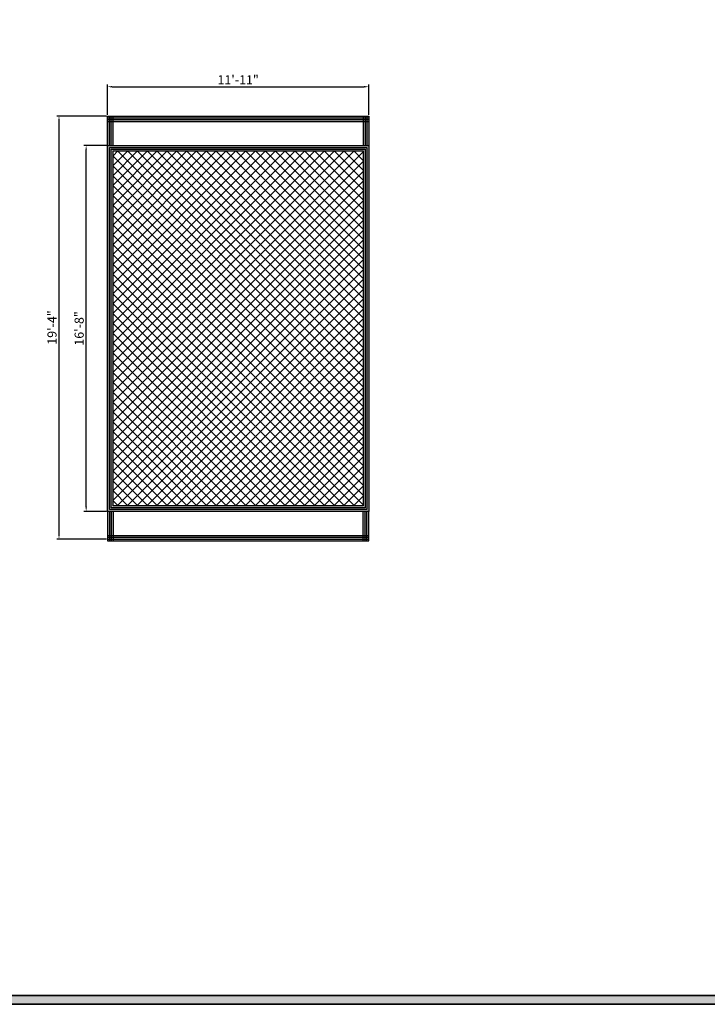
# Model space of a CAD drawing. Units: inches. Extents: x 1804 to 3296, y 909 to 2477.
# Tile 23 of 31: x 2543 to 2920, y 909 to 1449. Entities that reach past the tile are written whole.
import ezdxf

# ---------------------------------------------------------------- set-up
doc = ezdxf.new("R2010")
doc.units = ezdxf.units.IN
for name, color, linetype, lineweight in [('A-ANNO-DIMS', 2, 'Continuous', 18), ('A-ANNO-TTLB', 156, 'Continuous', 35), ('A-WALL-PATT', 10, 'Continuous', 13), ('C-PROP', 7, 'Continuous', 25), ('C-PROP-PATT', 85, 'Continuous', 13)]:
    doc.layers.add(name, color=color, linetype=linetype, lineweight=lineweight)
doc.styles.get("Standard").update_dxf_attribs({"font": 'arial.ttf'})
doc.dimstyles.new('ISO-25', dxfattribs={"dimtxt": 5, "dimasz": 2.5, "dimexe": 1.25, "dimexo": 0.625, "dimtad": 1, "dimdec": 0, "dimlunit": 4, "dimtxsty": 'Standard', "dimcen": 2.5, "dimadec": 0, "dimazin": 0, "dimtfac": 1, "dimtdec": 0, "dimtmove": 0, "dimatfit": 3, "dimfxl": 1, "dimarcsym": 0})

# ---------------------------------------------------------------- blocks, each defined once
blk = doc.blocks.new('*D40')
at = {"layer": 'A-ANNO-DIMS', "color": 0, "lineweight": -2, "transparency": 16777216}
for p, q in [((2590.91, 1395.84), (2563.72, 1395.84)), ((2564.97, 1166.73), (2564.97, 1393.34)), ((2590.91, 1164.23), (2563.72, 1164.23))]:
    blk.add_line(p, q, dxfattribs=at)
at = {"layer": 'A-ANNO-DIMS', "color": 0, "lineweight": 100, "transparency": 16777216}
for points in [[(2564.55, 1393.34), (2565.38, 1393.34), (2564.97, 1395.84)], [(2564.55, 1166.73), (2565.38, 1166.73), (2564.97, 1164.23)]]:
    blk.add_solid(points, dxfattribs=at)
at = {"layer": 'Defpoints', "color": 0, "lineweight": 100, "transparency": 16777216}
for p in [(2564.97, 1395.84), (2591.54, 1395.84), (2591.54, 1164.23)]:
    blk.add_point(p, dxfattribs=at)
at = {"layer": 'A-ANNO-DIMS', "color": 0, "transparency": 16777216, "insert": (2561.79, 1280.03), "char_height": 5, "attachment_point": 5, "rotation": 90}
blk.add_mtext('19\'-4"', dxfattribs=at)
blk = doc.blocks.new('*D41')
at = {"layer": 'A-ANNO-DIMS', "color": 0, "lineweight": -2, "transparency": 16777216}
for p, q in [((2590.91, 1379.68), (2578.58, 1379.68)), ((2579.83, 1181.88), (2579.83, 1377.18)), ((2590.91, 1179.38), (2578.58, 1179.38))]:
    blk.add_line(p, q, dxfattribs=at)
at = {"layer": 'A-ANNO-DIMS', "color": 0, "lineweight": 100, "transparency": 16777216}
for points in [[(2579.41, 1377.18), (2580.24, 1377.18), (2579.83, 1379.68)], [(2579.41, 1181.88), (2580.24, 1181.88), (2579.83, 1179.38)]]:
    blk.add_solid(points, dxfattribs=at)
at = {"layer": 'Defpoints', "color": 0, "lineweight": 100, "transparency": 16777216}
for p in [(2579.83, 1379.68), (2591.54, 1379.68), (2591.54, 1179.38)]:
    blk.add_point(p, dxfattribs=at)
at = {"layer": 'A-ANNO-DIMS', "color": 0, "transparency": 16777216, "insert": (2576.65, 1279.53), "char_height": 5, "attachment_point": 5, "rotation": 90}
blk.add_mtext('16\'-8"', dxfattribs=at)
blk = doc.blocks.new('*D42')
at = {"layer": 'A-ANNO-DIMS', "color": 0, "lineweight": -2, "transparency": 16777216}
for p, q in [((2591.54, 1396.47), (2591.54, 1413.1)), ((2734.5, 1396.47), (2734.5, 1413.1)), ((2594.04, 1411.85), (2732, 1411.85))]:
    blk.add_line(p, q, dxfattribs=at)
at = {"layer": 'A-ANNO-DIMS', "color": 0, "lineweight": 100, "transparency": 16777216}
for points in [[(2594.04, 1412.27), (2594.04, 1411.44), (2591.54, 1411.85)], [(2732, 1412.27), (2732, 1411.44), (2734.5, 1411.85)]]:
    blk.add_solid(points, dxfattribs=at)
at = {"layer": 'Defpoints', "color": 0, "lineweight": 100, "transparency": 16777216}
for p in [(2734.5, 1411.85), (2591.54, 1395.84), (2734.5, 1395.84)]:
    blk.add_point(p, dxfattribs=at)
at = {"layer": 'A-ANNO-DIMS', "color": 0, "transparency": 16777216, "insert": (2663.02, 1414.99), "char_height": 5, "attachment_point": 5}
blk.add_mtext('11\'-11"', dxfattribs=at)

msp = doc.modelspace()

# ---------------------------------------------------------------- hatches: boundary and pattern name
at = {"layer": 'A-ANNO-TTLB'}
h = msp.add_hatch(color=256, dxfattribs=at)
h.dxf.hatch_style = 1
h.paths.add_polyline_path([(3294.53, 2476.54), (1803.79, 2476.54), (1805.43, 909.47), (3296.17, 909.47)])
h.paths.add_polyline_path([(1811, 914.33), (1812.79, 2467.54), (3285.53, 2467.54), (3283.74, 914.33)], flags=16)
h.paths.add_polyline_path([(1925.58, 1062.77), (1925.58, 1138.07), (1925.58, 1539.88), (1925.58, 1793.38), (1925.58, 1830.04), (2325.54, 1830.04), (2325.54, 1793.38), (2325.54, 1586.42), (2325.54, 1138.07), (2325.54, 1062.77)], flags=0)
h.paths.add_polyline_path([(1997.22, 1029.4), (2008.85, 1037.96), (2008.85, 1020.84)], flags=0)
h.paths.add_polyline_path([(1934.58, 1138.07), (1934.58, 1147.07), (2078.77, 1147.07), (2078.77, 1138.07), (2060.94, 1138.07)], flags=0)
h.paths.add_polyline_path([(1944.35, 1138.07), (1944.35, 1147.07), (2056.05, 1147.07), (2056.05, 1138.07)], flags=0)
h.paths.add_polyline_path([(2222.24, 1037.96), (2233.87, 1029.4), (2222.24, 1020.84)], flags=0)
h.paths.add_polyline_path([(2061.94, 1139.07), (2061.94, 1146.07), (2077.77, 1146.07), (2077.77, 1139.07)], flags=0)
h.paths.add_polyline_path([(2149.58, 1138.07), (2149.58, 1269.44), (2158.58, 1269.44), (2158.58, 1326.69), (2149.58, 1326.69), (2149.58, 1340.94), (2139.6, 1340.94), (2139.6, 1434.25), (2149.58, 1434.25), (2149.58, 1447.36), (2158.58, 1447.36), (2158.58, 1423.87), (2158.58, 1408.06), (2198.46, 1408.06), (2198.46, 1412.56), (2282.65, 1412.56), (2282.65, 1465.94), (2316.54, 1465.94), (2316.54, 1590.92), (2192.86, 1590.92), (2192.86, 1595.3), (2291.17, 1595.3), (2291.17, 1590.92), (2316.54, 1590.92), (2316.54, 1784.38), (2300.24, 1784.38), (2300.24, 1757.47), (2268, 1757.47), (2268, 1681.04), (2180.87, 1681.04), (2180.87, 1757.47), (2148.63, 1757.47), (2148.63, 1784.38), (2119.08, 1784.38), (2119.08, 1585.58), (2114.58, 1585.58), (2114.58, 1784.38), (2064.11, 1784.38), (2046.28, 1784.38), (2046.28, 1760.38), (1958.58, 1760.38), (1958.58, 1664.38), (1934.58, 1664.38), (1934.58, 1784.38), (1934.58, 1793.38), (2046.28, 1793.38), (2064.11, 1793.38), (2119.08, 1793.38), (2230.78, 1793.38), (2230.78, 1784.38), (2268, 1784.38), (2300.24, 1784.38), (2316.54, 1784.38), (2316.54, 1590.92), (2316.54, 1373.73), (2316.54, 1138.07)], flags=0)
h.paths.add_polyline_path([(2209.19, 1166.63), (2209.19, 1175.63), (2158.58, 1175.63), (2209.19, 1223.63), (2209.19, 1231.63), (2183.88, 1231.63), (2183.88, 1301.66), (2242.59, 1301.66), (2242.59, 1326.69), (2316.54, 1326.69), (2272.59, 1271.63), (2272.59, 1223.63), (2316.54, 1175.63), (2272.59, 1175.63), (2272.59, 1166.63)], flags=0)
h.paths.add_polyline_path([(1947.77, 1345.22), (1947.77, 1457.48), (1991.2, 1457.48), (1991.2, 1451.7), (1991.2, 1352.18), (1991.2, 1345.22)], flags=0)
h.paths.add_polyline_path([(2209.19, 1271.63), (2262.59, 1271.63), (2262.59, 1311.85), (2272.59, 1301.66), (2272.59, 1271.63), (2269.92, 1269.63), (2270.59, 1269.63), (2270.59, 1225.63), (2211.19, 1225.63), (2211.19, 1269.63), (2211.86, 1269.63)], flags=0)
h.paths.add_polyline_path([(2000.34, 1378.21), (2000.34, 1429.71), (2025.22, 1429.71), (2025.22, 1378.21)], flags=0)
h.paths.add_polyline_path([(2001.34, 1379.21), (2001.34, 1428.71), (2024.22, 1428.71), (2024.22, 1379.21)], flags=0)
h.paths.add_polyline_path([(2012.34, 1390.21), (2012.34, 1417.71), (2013.22, 1417.71), (2013.22, 1390.21)], flags=0)
h.paths.add_polyline_path([(2237.56, 1331.19), (2237.56, 1340.18), (2238.62, 1340.18), (2238.62, 1386.84), (2241.04, 1386.84), (2242.06, 1386.84), (2242.06, 1408.06), (2316.54, 1331.19)], flags=0)
h.paths.add_polyline_path([(1953.73, 1464.35), (1953.73, 1498.59), (1981.74, 1498.59), (1981.74, 1464.35)], flags=0)
h.paths.add_polyline_path([(1987.63, 1462.08), (1987.63, 1500.95), (2104.07, 1500.95), (2104.07, 1462.08), (2099.27, 1462.08), (1993.6, 1462.08)], flags=0)
h.paths.add_polyline_path([(1956.06, 1481.47, -1), (1979.41, 1481.47, -1)], flags=0)
edge = h.paths.add_edge_path(flags=0)
edge.add_ellipse((2299.53, 1438.37), major_axis=(0.31, 21.36), ratio=0.670333, start_angle=0, end_angle=360)
h.paths.add_polyline_path([(2297.39, 1438.37, -1), (2301.67, 1438.37, -1)], flags=0)
h.paths.add_polyline_path([(2591.54, 1163.23), (2591.54, 1179.38), (2591.54, 1379.68), (2591.54, 1395.84), (2734.5, 1395.84), (2734.5, 1379.68), (2734.5, 1179.38), (2734.5, 1163.23)], flags=0)
h.paths.add_polyline_path([(2592.54, 1164.23), (2592.54, 1166.23), (2733.5, 1166.23), (2733.5, 1164.23)], flags=0)
h.paths.add_polyline_path([(2592.54, 1180.38), (2592.54, 1378.68), (2733.5, 1378.68), (2733.5, 1180.38)], flags=0)
h.paths.add_polyline_path([(2593.54, 1181.38), (2593.54, 1377.68), (2732.5, 1377.68), (2732.5, 1181.38)], flags=0)
h.paths.add_polyline_path([(2594.54, 1182.38), (2594.54, 1376.68), (2731.5, 1376.68), (2731.5, 1182.38)], flags=0)
h.paths.add_polyline_path([(1936.95, 1697.46), (1936.95, 1736.46), (1955.41, 1736.46), (1955.41, 1697.46)], flags=0)
h.paths.add_polyline_path([(1938.48, 1718.36), (1938.48, 1734.92), (1953.65, 1734.92), (1953.65, 1718.36)], flags=0)
h.paths.add_polyline_path([(1944.75, 1726.64, -1), (1947.37, 1726.64, -1)], flags=0)
h.paths.add_polyline_path([(2592.54, 1394.84), (2733.5, 1394.84), (2733.5, 1392.84), (2592.54, 1392.84)], flags=0)
h.paths.add_polyline_path([(1976.61, 1762.5), (1976.61, 1781.44), (2012.79, 1781.44), (2012.79, 1762.5)], flags=0)
h.paths.add_polyline_path([(1979.57, 1771.97, -1), (1991.39, 1771.97, -1)], flags=0)
h.paths.add_polyline_path([(1995.36, 1771.97, -1), (2007.18, 1771.97, -1)], flags=0)
h.paths.add_polyline_path([(2251.51, 1744.53), (2268, 1730.05), (2251.51, 1730.05)], flags=0)
h.paths.add_polyline_path([(2047.28, 1785.38), (2047.28, 1792.38), (2063.11, 1792.38), (2063.11, 1785.38)], flags=0)
h.paths.add_polyline_path([(2155.08, 1770.92, -1), (2174.42, 1770.92, -1)], flags=0)
h.paths.add_polyline_path([(2188.59, 1758.27), (2188.59, 1772.81), (2222.3, 1772.81), (2222.3, 1758.27)], flags=0)
h.paths.add_polyline_path([(2223.97, 1758.27), (2223.97, 1772.81), (2257.68, 1772.81), (2257.68, 1758.27)], flags=0)
h.paths.add_polyline_path([(2274.45, 1770.92, -1), (2293.8, 1770.92, -1)], flags=0)
h.paths.add_polyline_path([(2591.54, 1582.09), (2591.54, 1782.39), (2734.5, 1782.39), (2734.5, 1582.09)], flags=0)
h.paths.add_polyline_path([(2592.54, 1583.09), (2592.54, 1781.39), (2733.5, 1781.39), (2733.5, 1583.09)], flags=0)
h.paths.add_polyline_path([(2593.54, 1584.09), (2593.54, 1780.39), (2732.5, 1780.39), (2732.5, 1584.09)], flags=0)
h.paths.add_polyline_path([(2594.54, 1585.09), (2594.54, 1779.39), (2731.5, 1779.39), (2731.5, 1585.09)], flags=0)
h.paths.add_polyline_path([(1922.17, 1978.79), (1922.17, 2295.08), (1922.17, 2296.08), (2115.67, 2296.08), (2115.67, 2384.31), (2115.67, 2385.31), (2322.12, 2385.31), (2323.12, 2385.31), (2323.12, 1979.79), (2323.12, 1978.79), (1923.17, 1978.79)], flags=0)
h.paths.add_polyline_path([(1922.17, 1978.79), (1922.17, 2051.31), (1922.17, 2214.86), (1922.17, 2296.08), (2115.67, 2296.08), (2115.67, 2385.31), (2323.12, 2385.31), (2323.12, 2280.42), (2323.12, 1978.79), (2115.67, 1978.79)], flags=0)
h.paths.add_polyline_path([(1923.17, 1979.79), (1923.17, 2050.31), (2115.67, 2050.31), (2115.67, 2051.31), (1923.17, 2051.31), (1923.17, 2213.86), (1923.17, 2214.86), (1923.17, 2295.08), (1990.02, 2295.08), (1990.02, 2214.86), (1991.02, 2214.86), (1991.02, 2295.08), (2115.67, 2295.08), (2115.67, 1979.79), (2116.67, 1979.79), (2116.67, 2304.18), (2116.67, 2384.31), (2322.12, 2384.31), (2322.12, 2280.42), (2322.12, 1979.79), (2115.67, 1979.79)], flags=0)
h.paths.add_polyline_path([(2972.46, 1192.5), (2972.46, 1196.92), (2995.47, 1196.92), (2995.47, 1255.47), (2995.09, 1255.47), (2987.42, 1249.39), (2980.08, 1255.47), (2978.05, 1255.47), (2978.05, 1257.24), (2995.47, 1257.24), (2995.47, 1261.58), (3015.37, 1261.58), (3015.37, 1333.28), (3015.37, 1414.4), (3032.82, 1414.4), (3032.82, 1333.28), (3032.82, 1261.58), (3052.66, 1261.58), (3052.66, 1255.47), (3079.86, 1255.47), (3078.72, 1254.57), (3081.47, 1252.29), (3078.56, 1249.99), (3075.81, 1252.26), (3072.57, 1249.69), (3070.36, 1251.52), (3067.67, 1249.39), (3060.34, 1255.47), (3052.66, 1255.47), (3052.66, 1196.92), (3054.58, 1196.92), (3074, 1196.92), (3074, 1192.5), (3052.66, 1192.5), (2995.47, 1192.5)], flags=0)
h.paths.add_polyline_path([(2490.75, 1979.27), (2490.75, 1980.27), (2596.87, 1980.27), (2596.87, 2051.8), (2596.87, 2052.8), (2596.87, 2216.35), (2596.87, 2297.57), (2717.32, 2297.57), (2710.57, 2305.62), (2724.07, 2305.62), (2717.32, 2297.57), (2782.37, 2297.57), (2782.37, 2395.8), (3006.82, 2395.8), (3006.82, 1981.27), (3093.73, 1981.27), (3093.73, 1980.27), (3047.51, 1980.27), (3046.37, 1979.37), (3049.11, 1977.1), (3046.2, 1974.79), (3043.46, 1977.07), (3040.21, 1974.49), (3038, 1976.32), (3035.32, 1974.2), (3027.98, 1980.27), (2871.83, 1980.27), (2871.83, 1981.27), (2791.37, 1981.27), (2791.37, 2050.8), (2597.87, 2050.8), (2597.87, 1980.27), (2597.87, 1979.27), (2546.27, 1979.27), (2545.12, 1978.37), (2547.87, 1976.1), (2544.96, 1973.79), (2542.22, 1976.07), (2538.97, 1973.49), (2536.76, 1975.32), (2534.07, 1973.2), (2526.74, 1979.27)], flags=0)
h.paths.add_polyline_path([(2597.87, 2051.8), (2606.87, 2051.8), (2606.87, 2258.39), (2597.87, 2258.39), (2597.87, 2296.57), (2606.87, 2296.57), (2606.87, 2262.39), (2782.37, 2262.39), (2782.37, 2296.57), (2790.37, 2296.57), (2790.37, 2262.39), (2791.37, 2262.39), (2791.37, 2305.67), (2791.37, 2385.8), (2996.82, 2385.8), (2996.82, 2339.85), (3006.82, 2339.85), (3006.82, 2250.12), (2997.82, 2250.12), (2997.82, 1981.27), (2996.82, 1981.27), (2872.83, 1981.27), (2872.83, 1991.8), (2871.83, 1991.8), (2871.83, 2050.8), (2790.37, 2050.8), (2597.87, 2050.8)], flags=0)
h.paths.add_polyline_path([(2179.93, 2153.92), (2179.93, 2353.97), (2259.98, 2353.97), (2259.98, 2153.92)], flags=0)
h.paths.add_polyline_path([(2180.93, 2154.92), (2180.93, 2352.97), (2258.98, 2352.97), (2258.98, 2154.92)], flags=0)
h.paths.add_polyline_path([(2960.87, 1608.49), (2960.87, 1753.62), (3070.9, 1753.62), (3070.9, 1608.49)], flags=0)
h.paths.add_polyline_path([(2961.87, 1609.49), (2961.87, 1752.62), (3069.9, 1752.62), (3069.9, 1609.49)], flags=0)
h.paths.add_polyline_path([(2962.87, 1610.49), (2962.87, 1751.62), (3068.9, 1751.62), (3068.9, 1610.49)], flags=0)
h.paths.add_polyline_path([(2963.87, 1611.49), (2963.87, 1750.62), (3067.9, 1750.62), (3067.9, 1611.49)], flags=0)
h.paths.add_polyline_path([(2782.37, 2051.8), (2782.37, 2216.32), (2791.37, 2216.32), (2791.37, 2051.8), (2872.83, 2051.8), (2872.83, 2068.56), (2884.67, 2068.56), (2884.67, 2085.33), (2896.51, 2085.33), (2896.51, 2102.09), (2908.36, 2102.09), (2908.36, 2118.85), (2920.2, 2118.85), (2920.2, 2135.62), (2932.05, 2135.62), (2932.05, 2145.3), (2925.08, 2145.3), (2925.08, 2203.2), (2996.82, 2203.2), (2996.82, 2145.3), (2953.82, 2145.3), (2872.83, 2051.8), (2790.37, 2051.8)], flags=0)
h.paths.add_polyline_path([(2717.32, 2238.65), (2710.57, 2246.7), (2724.07, 2246.7)], flags=0)
h.paths.add_polyline_path([(2003.09, 1122.79), (2017.16, 1122.79), (2017.16, 1138.74), (2003.09, 1138.74)], flags=8)
h.paths.add_polyline_path([(2174.76, 1792.72), (2188.83, 1792.72), (2188.83, 1808.66), (2174.76, 1808.66)], flags=8)
h.paths.add_polyline_path([(1987.95, 1792.51), (2002.02, 1792.51), (2002.02, 1808.45), (1987.95, 1808.45)], flags=8)
h.paths.add_polyline_path([(2148.79, 1289.26), (2160.46, 1289.26), (2160.46, 1305.2), (2148.79, 1305.2)], flags=8)
h.paths.add_polyline_path([(2115.36, 1133.57), (2127.04, 1133.57), (2127.04, 1149.51), (2115.36, 1149.51)], flags=8)
h.paths.add_polyline_path([(2237.58, 1421.48), (2249.25, 1421.48), (2249.25, 1437.43), (2237.58, 1437.43)], flags=8)
h.paths.add_polyline_path([(2134.99, 1584.32), (2146.66, 1584.32), (2146.66, 1600.26), (2134.99, 1600.26)], flags=8)
h.paths.add_polyline_path([(2101.95, 1557.31), (2113.62, 1557.31), (2113.62, 1573.25), (2101.95, 1573.25)], flags=8)
h.paths.add_polyline_path([(2937.85, 1156.77), (3120.41, 1156.77), (3120.41, 1185.72), (2937.85, 1185.72)], flags=8)
h.paths.add_polyline_path([(2980.71, 1786.71), (3050.06, 1786.71), (3050.06, 1802.66), (2980.71, 1802.66)], flags=8)
h.paths.add_polyline_path([(2869.28, 1661.96), (2938.62, 1661.96), (2938.62, 1690.8), (2869.28, 1690.8)], flags=8)
h.paths.add_polyline_path([(3092.27, 1674.86), (3161.62, 1674.86), (3161.62, 1690.8), (3092.27, 1690.8)], flags=8)
h.paths.add_polyline_path([(2980.71, 1674.86), (3050.06, 1674.86), (3050.06, 1690.8), (2980.71, 1690.8)], flags=8)
h.paths.add_polyline_path([(2649.07, 1678.23), (2674.53, 1678.23), (2674.53, 1714.76), (2649.07, 1714.76)], flags=8)
h.paths.add_polyline_path([(2530.84, 1981.63), (2549.13, 1981.63), (2549.13, 1997.57), (2530.84, 1997.57)], flags=8)
h.paths.add_polyline_path([(3031.29, 1981.77), (3049.58, 1981.77), (3049.58, 1997.71), (3031.29, 1997.71)], flags=8)
h.paths.add_polyline_path([(2715.38, 1911.9), (2851.54, 1911.9), (2851.54, 1940.85), (2715.38, 1940.85)], flags=8)
h.paths.add_polyline_path([(2015.23, 1927.36), (2205.42, 1927.36), (2205.42, 1956.3), (2015.23, 1956.3)], flags=8)
h.paths.add_polyline_path([(2671.84, 2057.84), (2702.75, 2057.84), (2702.75, 2073.79), (2671.84, 2073.79)], flags=8)
h.paths.add_polyline_path([(2678.5, 2316.52), (2765.26, 2316.52), (2765.26, 2332.46), (2678.5, 2332.46)], flags=8)
h.paths.add_polyline_path([(2678.48, 2271.96), (2736.41, 2271.96), (2736.41, 2287.9), (2678.48, 2287.9)], flags=8)
h.paths.add_polyline_path([(2019.2, 972.79), (2243.21, 972.79), (2243.21, 1001.74), (2019.2, 1001.74)], flags=8)
h.paths.add_polyline_path([(2097.06, 1021.56), (2132.16, 1021.56), (2132.16, 1037.51), (2097.06, 1037.51)], flags=8)
h.paths.add_polyline_path([(2182.47, 1360.48), (2207.35, 1360.48), (2207.35, 1376.42), (2182.47, 1376.42)], flags=8)
h.paths.add_polyline_path([(2261.12, 1361.77), (2295.01, 1361.77), (2295.01, 1377.71), (2261.12, 1377.71)], flags=8)
h.paths.add_polyline_path([(2245.75, 1511.51), (2278.44, 1511.51), (2278.44, 1527.46), (2245.75, 1527.46)], flags=8)
h.paths.add_polyline_path([(1991.16, 1296.29), (2060.51, 1296.29), (2060.51, 1312.23), (1991.16, 1312.23)], flags=8)
h.paths.add_polyline_path([(2187, 1651.35), (2246.71, 1651.35), (2246.71, 1667.29), (2187, 1667.29)], flags=8)
h.paths.add_polyline_path([(1976.49, 1684.81), (2068.63, 1684.81), (2068.63, 1700.76), (1976.49, 1700.76)], flags=8)
at = {"layer": 'A-WALL-PATT'}
h = msp.add_hatch(color=256, dxfattribs=at)
h.dxf.hatch_style = 1
h.paths.add_polyline_path([(2158.58, 1275.49), (2155.29, 1275.49), (2149.58, 1275.49), (2149.58, 1269.44), (2158.58, 1269.44)])
h.paths.add_polyline_path([(2158.58, 1326.69), (2149.58, 1326.69), (2149.58, 1319.33), (2155.29, 1319.33), (2158.58, 1319.33)])
h.paths.add_polyline_path([(2158.58, 1402.2), (2158.58, 1423.87), (2158.58, 1447.36), (2149.58, 1447.36), (2149.58, 1423.87), (2149.58, 1340.94), (2149.58, 1326.69), (2158.58, 1326.69), (2158.58, 1354.23)])
h.paths.add_polyline_path([(1965.87, 1658.79), (1965.87, 1679.09), (1955.57, 1679.09), (1955.57, 1658.79)], flags=9)
h.paths.add_polyline_path([(2293.18, 1677.29), (2293.18, 1697.58), (2282.88, 1697.58), (2282.88, 1677.29)], flags=9)
h.paths.add_polyline_path([(2271.13, 1545.23), (2287.53, 1545.23), (2287.53, 1555.53), (2271.13, 1555.53)], flags=9)
h.paths.add_polyline_path([(2303.26, 1488.52), (2303.26, 1508.82), (2292.95, 1508.82), (2292.95, 1488.52)], flags=9)
h.paths.add_polyline_path([(2271.13, 1393.15), (2287.53, 1393.15), (2287.53, 1403.45), (2271.13, 1403.45)], flags=9)
h.paths.add_polyline_path([(2306.48, 1361.45), (2306.48, 1377.86), (2296.18, 1377.86), (2296.18, 1361.45)], flags=9)
h.paths.add_polyline_path([(2189.9, 1340.62), (2206.31, 1340.62), (2206.31, 1350.92), (2189.9, 1350.92)], flags=9)
h.paths.add_polyline_path([(2174.54, 1361.45), (2174.54, 1377.86), (2164.23, 1377.86), (2164.23, 1361.45)], flags=9)
h.paths.add_polyline_path([(2304.24, 1240.8), (2304.24, 1261.09), (2293.94, 1261.09), (2293.94, 1240.8)], flags=9)
h.paths.add_polyline_path([(2227.19, 1188.73), (2247.49, 1188.73), (2247.49, 1199.03), (2227.19, 1199.03)], flags=9)
h.paths.add_polyline_path([(2181.93, 1144.21), (2181.93, 1160.62), (2171.63, 1160.62), (2171.63, 1144.21)], flags=9)
h.paths.add_polyline_path([(1968.21, 1333.34), (1968.21, 1353.64), (1957.91, 1353.64), (1957.91, 1333.34)], flags=9)
h.paths.add_polyline_path([(2029.78, 1203.53), (2053.95, 1203.53), (2053.95, 1213.83), (2029.78, 1213.83)], flags=9)
h.paths.add_polyline_path([(2576.51, 1671.88), (2576.51, 1692.17), (2566.21, 1692.17), (2566.21, 1671.88)], flags=9)
h.paths.add_polyline_path([(2566.99, 1269.67), (2566.99, 1289.96), (2556.68, 1289.96), (2556.68, 1269.67)], flags=9)
h.paths.add_polyline_path([(2581.85, 1269.17), (2581.85, 1289.46), (2571.54, 1289.46), (2571.54, 1269.17)], flags=9)
h.paths.add_polyline_path([(2650.71, 1409.75), (2674.89, 1409.75), (2674.89, 1420.05), (2650.71, 1420.05)], flags=9)
h.paths.add_polyline_path([(2003.09, 1122.79), (2017.16, 1122.79), (2017.16, 1138.74), (2003.09, 1138.74)], flags=9)
h.paths.add_polyline_path([(2174.76, 1792.72), (2188.83, 1792.72), (2188.83, 1808.66), (2174.76, 1808.66)], flags=9)
h.paths.add_polyline_path([(1987.95, 1792.51), (2002.02, 1792.51), (2002.02, 1808.45), (1987.95, 1808.45)], flags=9)
h.paths.add_polyline_path([(2148.79, 1289.26), (2160.46, 1289.26), (2160.46, 1305.2), (2148.79, 1305.2)], flags=9)
h.paths.add_polyline_path([(2115.36, 1133.57), (2127.04, 1133.57), (2127.04, 1149.51), (2115.36, 1149.51)], flags=9)
h.paths.add_polyline_path([(2237.58, 1421.48), (2249.25, 1421.48), (2249.25, 1437.43), (2237.58, 1437.43)], flags=9)
h.paths.add_polyline_path([(2134.99, 1584.32), (2146.66, 1584.32), (2146.66, 1600.26), (2134.99, 1600.26)], flags=9)
h.paths.add_polyline_path([(2101.95, 1557.31), (2113.62, 1557.31), (2113.62, 1573.25), (2101.95, 1573.25)], flags=9)
h.paths.add_polyline_path([(2937.85, 1156.77), (3120.41, 1156.77), (3120.41, 1185.72), (2937.85, 1185.72)], flags=9)
h.paths.add_polyline_path([(2980.71, 1786.71), (3050.06, 1786.71), (3050.06, 1802.66), (2980.71, 1802.66)], flags=9)
h.paths.add_polyline_path([(2869.28, 1661.96), (2938.62, 1661.96), (2938.62, 1690.8), (2869.28, 1690.8)], flags=9)
h.paths.add_polyline_path([(3092.27, 1674.86), (3161.62, 1674.86), (3161.62, 1690.8), (3092.27, 1690.8)], flags=9)
h.paths.add_polyline_path([(2980.71, 1674.86), (3050.06, 1674.86), (3050.06, 1690.8), (2980.71, 1690.8)], flags=9)
h.paths.add_polyline_path([(2649.07, 1678.23), (2674.53, 1678.23), (2674.53, 1714.76), (2649.07, 1714.76)], flags=9)
h.paths.add_polyline_path([(2530.84, 1981.63), (2549.13, 1981.63), (2549.13, 1997.57), (2530.84, 1997.57)], flags=9)
h.paths.add_polyline_path([(3031.29, 1981.77), (3049.58, 1981.77), (3049.58, 1997.71), (3031.29, 1997.71)], flags=9)
h.paths.add_polyline_path([(2715.38, 1911.9), (2851.54, 1911.9), (2851.54, 1940.85), (2715.38, 1940.85)], flags=9)
h.paths.add_polyline_path([(2015.23, 1927.36), (2205.42, 1927.36), (2205.42, 1956.3), (2015.23, 1956.3)], flags=9)
h.paths.add_polyline_path([(2671.84, 2057.84), (2702.75, 2057.84), (2702.75, 2073.79), (2671.84, 2073.79)], flags=9)
h.paths.add_polyline_path([(2678.5, 2316.52), (2765.26, 2316.52), (2765.26, 2332.46), (2678.5, 2332.46)], flags=9)
h.paths.add_polyline_path([(2678.48, 2271.96), (2736.41, 2271.96), (2736.41, 2287.9), (2678.48, 2287.9)], flags=9)
h.paths.add_polyline_path([(2019.2, 972.79), (2243.21, 972.79), (2243.21, 1001.74), (2019.2, 1001.74)], flags=9)
h.paths.add_polyline_path([(2097.06, 1021.56), (2132.16, 1021.56), (2132.16, 1037.51), (2097.06, 1037.51)], flags=9)
h.paths.add_polyline_path([(2182.47, 1360.48), (2207.35, 1360.48), (2207.35, 1376.42), (2182.47, 1376.42)], flags=9)
h.paths.add_polyline_path([(2261.12, 1361.77), (2295.01, 1361.77), (2295.01, 1377.71), (2261.12, 1377.71)], flags=9)
h.paths.add_polyline_path([(2245.75, 1511.51), (2278.44, 1511.51), (2278.44, 1527.46), (2245.75, 1527.46)], flags=9)
h.paths.add_polyline_path([(1991.16, 1296.29), (2060.51, 1296.29), (2060.51, 1312.23), (1991.16, 1312.23)], flags=9)
h.paths.add_polyline_path([(2187, 1651.35), (2246.71, 1651.35), (2246.71, 1667.29), (2187, 1667.29)], flags=9)
h.paths.add_polyline_path([(1976.49, 1684.81), (2068.63, 1684.81), (2068.63, 1700.76), (1976.49, 1700.76)], flags=9)
at = {"layer": 'C-PROP-PATT'}
h = msp.add_hatch(color=256, dxfattribs=at)
h.dxf.hatch_style = 1
h.paths.add_polyline_path([(2734.5, 1392.84), (2733.5, 1392.84), (2733.5, 1379.68), (2734.5, 1379.68)])
h.paths.add_polyline_path([(2733.5, 1392.84), (2732.5, 1392.84), (2732.5, 1379.68), (2733.5, 1379.68)])
h.paths.add_polyline_path([(2732.5, 1392.84), (2731.5, 1392.84), (2731.5, 1379.68), (2732.5, 1379.68)])
h.paths.add_polyline_path([(2734.5, 1379.68), (2733.5, 1379.68), (2732.5, 1379.68), (2731.5, 1379.68), (2591.54, 1379.68), (2591.54, 1179.38), (2734.5, 1179.38)])
h.paths.add_polyline_path([(2733.5, 1180.38), (2592.54, 1180.38), (2592.54, 1378.68), (2733.5, 1378.68)], flags=16)
h.paths.add_polyline_path([(2732.5, 1181.38), (2593.54, 1181.38), (2593.54, 1377.68), (2732.5, 1377.68)], flags=0)
h.paths.add_polyline_path([(2731.5, 1182.38), (2594.54, 1182.38), (2594.54, 1376.68), (2731.5, 1376.68)], flags=0)
h.paths.add_polyline_path([(2732.5, 1377.68), (2593.54, 1377.68), (2593.54, 1181.38), (2732.5, 1181.38)], flags=0)
h.paths.add_polyline_path([(2731.5, 1394.84), (2594.54, 1394.84), (2594.54, 1393.84), (2731.5, 1393.84)])
h.paths.add_polyline_path([(2731.5, 1393.84), (2594.54, 1393.84), (2594.54, 1392.84), (2731.5, 1392.84)])
h.paths.add_polyline_path([(2731.5, 1395.84), (2594.54, 1395.84), (2594.54, 1394.84), (2731.5, 1394.84)])
h.paths.add_polyline_path([(2733.5, 1393.84), (2732.5, 1393.84), (2732.5, 1392.84), (2733.5, 1392.84)])
h.paths.add_polyline_path([(2734.5, 1393.84), (2733.5, 1393.84), (2733.5, 1392.84), (2734.5, 1392.84)])
h.paths.add_polyline_path([(2733.5, 1394.84), (2732.5, 1394.84), (2732.5, 1393.84), (2733.5, 1393.84)])
h.paths.add_polyline_path([(2732.5, 1393.84), (2731.5, 1393.84), (2731.5, 1392.84), (2732.5, 1392.84)])
h.paths.add_polyline_path([(2732.5, 1394.84), (2731.5, 1394.84), (2731.5, 1393.84), (2732.5, 1393.84)])
h.paths.add_polyline_path([(2732.5, 1395.84), (2731.5, 1395.84), (2731.5, 1394.84), (2732.5, 1394.84)])
h.paths.add_polyline_path([(2733.5, 1395.84), (2732.5, 1395.84), (2732.5, 1394.84), (2733.5, 1394.84)])
h.paths.add_polyline_path([(2734.5, 1394.84), (2733.5, 1394.84), (2733.5, 1393.84), (2734.5, 1393.84)])
h.paths.add_polyline_path([(2734.5, 1395.84), (2733.5, 1395.84), (2733.5, 1394.84), (2734.5, 1394.84)])
h.paths.add_polyline_path([(2592.54, 1393.84), (2591.54, 1393.84), (2591.54, 1392.84), (2592.54, 1392.84)])
h.paths.add_polyline_path([(2592.54, 1394.84), (2591.54, 1394.84), (2591.54, 1393.84), (2592.54, 1393.84)])
h.paths.add_polyline_path([(2593.54, 1393.84), (2592.54, 1393.84), (2592.54, 1392.84), (2593.54, 1392.84)])
h.paths.add_polyline_path([(2593.54, 1394.84), (2592.54, 1394.84), (2592.54, 1393.84), (2593.54, 1393.84)])
h.paths.add_polyline_path([(2592.54, 1395.84), (2591.54, 1395.84), (2591.54, 1394.84), (2592.54, 1394.84)])
h.paths.add_polyline_path([(2593.54, 1395.84), (2592.54, 1395.84), (2592.54, 1394.84), (2593.54, 1394.84)])
h.paths.add_polyline_path([(2594.54, 1394.84), (2593.54, 1394.84), (2593.54, 1393.84), (2594.54, 1393.84)])
h.paths.add_polyline_path([(2594.54, 1393.84), (2593.54, 1393.84), (2593.54, 1392.84), (2594.54, 1392.84)])
h.paths.add_polyline_path([(2594.54, 1392.84), (2593.54, 1392.84), (2593.54, 1379.68), (2594.54, 1379.68)])
h.paths.add_polyline_path([(2594.54, 1395.84), (2593.54, 1395.84), (2593.54, 1394.84), (2594.54, 1394.84)])
h.paths.add_polyline_path([(2593.54, 1392.84), (2592.54, 1392.84), (2592.54, 1379.68), (2593.54, 1379.68)])
h.paths.add_polyline_path([(2592.54, 1392.84), (2591.54, 1392.84), (2591.54, 1379.68), (2592.54, 1379.68)])
h.paths.add_polyline_path([(2592.54, 1166.23), (2591.54, 1166.23), (2591.54, 1165.23), (2592.54, 1165.23)])
h.paths.add_polyline_path([(2592.54, 1165.23), (2591.54, 1165.23), (2591.54, 1164.23), (2592.54, 1164.23)])
h.paths.add_polyline_path([(2592.54, 1164.23), (2591.54, 1164.23), (2591.54, 1163.23), (2592.54, 1163.23)])
h.paths.add_polyline_path([(2593.54, 1164.23), (2592.54, 1164.23), (2592.54, 1163.23), (2593.54, 1163.23)])
h.paths.add_polyline_path([(2593.54, 1165.23), (2592.54, 1165.23), (2592.54, 1164.23), (2593.54, 1164.23)])
h.paths.add_polyline_path([(2593.54, 1166.23), (2592.54, 1166.23), (2592.54, 1165.23), (2593.54, 1165.23)])
h.paths.add_polyline_path([(2594.54, 1165.23), (2593.54, 1165.23), (2593.54, 1164.23), (2594.54, 1164.23)])
h.paths.add_polyline_path([(2594.54, 1164.23), (2593.54, 1164.23), (2593.54, 1163.23), (2594.54, 1163.23)])
h.paths.add_polyline_path([(2594.54, 1179.38), (2593.54, 1179.38), (2593.54, 1166.23), (2594.54, 1166.23)])
h.paths.add_polyline_path([(2592.54, 1179.38), (2591.54, 1179.38), (2591.54, 1166.23), (2592.54, 1166.23)])
h.paths.add_polyline_path([(2593.54, 1179.38), (2592.54, 1179.38), (2592.54, 1166.23), (2593.54, 1166.23)])
h.paths.add_polyline_path([(2594.54, 1166.23), (2593.54, 1166.23), (2593.54, 1165.23), (2594.54, 1165.23)])
h.paths.add_polyline_path([(2734.5, 1179.38), (2733.5, 1179.38), (2733.5, 1166.23), (2734.5, 1166.23)])
h.paths.add_polyline_path([(2732.5, 1179.38), (2731.5, 1179.38), (2731.5, 1166.23), (2732.5, 1166.23)])
h.paths.add_polyline_path([(2733.5, 1179.38), (2732.5, 1179.38), (2732.5, 1166.23), (2733.5, 1166.23)])
h = msp.add_hatch(color=256, dxfattribs=at)
h.dxf.hatch_style = 1
h.paths.add_polyline_path([(2593.54, 1181.38), (2732.5, 1181.38), (2732.5, 1377.68), (2593.54, 1377.68)], flags=16)
h.paths.add_polyline_path([(2594.54, 1182.38), (2731.5, 1182.38), (2731.5, 1376.68), (2594.54, 1376.68)], flags=0)
h.paths.add_polyline_path([(2592.54, 1180.38), (2733.5, 1180.38), (2733.5, 1378.68), (2592.54, 1378.68)])
h = msp.add_hatch(color=256, dxfattribs=at)
h.dxf.hatch_style = 1
h.paths.add_polyline_path([(2732.5, 1377.68), (2593.54, 1377.68), (2593.54, 1181.38), (2732.5, 1181.38)])
h.paths.add_polyline_path([(2731.5, 1376.68), (2731.5, 1182.38), (2594.54, 1182.38), (2594.54, 1376.68)], flags=16)
h.paths.add_polyline_path([(2731.5, 1166.23), (2594.54, 1166.23), (2594.54, 1165.23), (2731.5, 1165.23)])
h.paths.add_polyline_path([(2731.5, 1164.23), (2594.54, 1164.23), (2594.54, 1163.23), (2731.5, 1163.23)])
h.paths.add_polyline_path([(2731.5, 1165.23), (2594.54, 1165.23), (2594.54, 1164.23), (2731.5, 1164.23)])
h.paths.add_polyline_path([(2732.5, 1166.23), (2731.5, 1166.23), (2731.5, 1165.23), (2732.5, 1165.23)])
h.paths.add_polyline_path([(2734.5, 1166.23), (2733.5, 1166.23), (2733.5, 1165.23), (2734.5, 1165.23)])
h.paths.add_polyline_path([(2732.5, 1165.23), (2731.5, 1165.23), (2731.5, 1164.23), (2732.5, 1164.23)])
h.paths.add_polyline_path([(2733.5, 1166.23), (2732.5, 1166.23), (2732.5, 1165.23), (2733.5, 1165.23)])
h.paths.add_polyline_path([(2733.5, 1165.23), (2732.5, 1165.23), (2732.5, 1164.23), (2733.5, 1164.23)])
h.paths.add_polyline_path([(2732.5, 1164.23), (2731.5, 1164.23), (2731.5, 1163.23), (2732.5, 1163.23)])
h.paths.add_polyline_path([(2733.5, 1164.23), (2732.5, 1164.23), (2732.5, 1163.23), (2733.5, 1163.23)])
h.paths.add_polyline_path([(2734.5, 1164.23), (2733.5, 1164.23), (2733.5, 1163.23), (2734.5, 1163.23)])
h.paths.add_polyline_path([(2734.5, 1165.23), (2733.5, 1165.23), (2733.5, 1164.23), (2734.5, 1164.23)])
h = msp.add_hatch(dxfattribs=at)
h.set_pattern_fill('ANSI37', color=256, scale=1.2)
h.set_pattern_definition([(45, (0, 293.5775), (-2.694077, 2.694077), []), (135, (0, 293.5775), (-2.694077, -2.694077), [])])
h.paths.add_polyline_path([(2731.5, 1376.68), (2594.54, 1376.68), (2594.54, 1182.38), (2731.5, 1182.38)])

# ---------------------------------------------------------------- linework, layer by layer
at = {"layer": 'A-ANNO-TTLB'}
for points in [[(1803.79, 2476.54), (3294.53, 2476.54), (3296.17, 909.47), (1805.43, 909.47)], [(1812.79, 2467.54), (3285.53, 2467.54), (3283.74, 914.33), (1811, 914.33)]]:
    msp.add_lwpolyline(points, close=True, dxfattribs=at)
at = {"layer": 'C-PROP'}
for p, q in [((2591.54, 1379.68), (2591.54, 1395.84)), ((2591.54, 1395.84), (2734.5, 1395.84)), ((2591.54, 1394.84), (2734.5, 1394.84)), ((2591.54, 1393.84), (2734.5, 1393.84)), ((2591.54, 1392.84), (2734.5, 1392.84)), ((2592.54, 1379.68), (2592.54, 1395.84)), ((2593.54, 1379.68), (2593.54, 1395.84)), ((2594.54, 1379.68), (2594.54, 1395.84)), ((2731.5, 1395.84), (2731.5, 1379.68)), ((2732.5, 1395.84), (2732.5, 1379.68)), ((2733.5, 1395.84), (2733.5, 1379.68)), ((2734.5, 1395.84), (2734.5, 1379.68)), ((2591.54, 1179.38), (2591.54, 1163.23)), ((2592.54, 1179.38), (2592.54, 1163.23)), ((2593.54, 1179.38), (2593.54, 1163.23)), ((2594.54, 1179.38), (2594.54, 1163.23)), ((2731.5, 1163.23), (2731.5, 1179.38)), ((2732.5, 1163.23), (2732.5, 1179.38)), ((2733.5, 1163.23), (2733.5, 1179.38)), ((2734.5, 1163.23), (2734.5, 1179.38)), ((2591.54, 1166.23), (2734.5, 1166.23)), ((2591.54, 1165.23), (2734.5, 1165.23)), ((2591.54, 1164.23), (2734.5, 1164.23)), ((2591.54, 1163.23), (2734.5, 1163.23))]:
    msp.add_line(p, q, dxfattribs=at)
for points in [[(2591.54, 1379.68), (2734.5, 1379.68), (2734.5, 1179.38), (2591.54, 1179.38)], [(2592.54, 1378.68), (2733.5, 1378.68), (2733.5, 1180.38), (2592.54, 1180.38)], [(2593.54, 1377.68), (2732.5, 1377.68), (2732.5, 1181.38), (2593.54, 1181.38)], [(2594.54, 1376.68), (2731.5, 1376.68), (2731.5, 1182.38), (2594.54, 1182.38)]]:
    msp.add_lwpolyline(points, close=True, dxfattribs=at)

# ---------------------------------------------------------------- dimensions: what is measured, and where the dimension line sits
at = {"layer": 'A-ANNO-DIMS'}
dim = msp.add_linear_dim(base=(2734.5, 1411.85), p1=(2591.54, 1395.84), p2=(2734.5, 1395.84), dimstyle='ISO-25', override={"dimclrd": 0, "dimclre": 0, "dimclrt": 0}, dxfattribs=at)
dim.commit()
dim.dimension.update_dxf_attribs({"geometry": '*D42', "text_midpoint": (2663.02, 1414.99)})
for base, p1, p2, picture, middle in [((2564.97, 1395.84), (2591.54, 1164.23), (2591.54, 1395.84), '*D40', (2561.79, 1280.03)), ((2579.83, 1379.68), (2591.54, 1179.38), (2591.54, 1379.68), '*D41', (2576.65, 1279.53))]:
    dim = msp.add_linear_dim(base=base, p1=p1, p2=p2, angle=90, dimstyle='ISO-25', override={"dimclrd": 0, "dimclre": 0, "dimclrt": 0}, dxfattribs=at)
    dim.commit()
    dim.dimension.update_dxf_attribs({"geometry": picture, "text_midpoint": middle})

doc.saveas('drawing.dxf')
